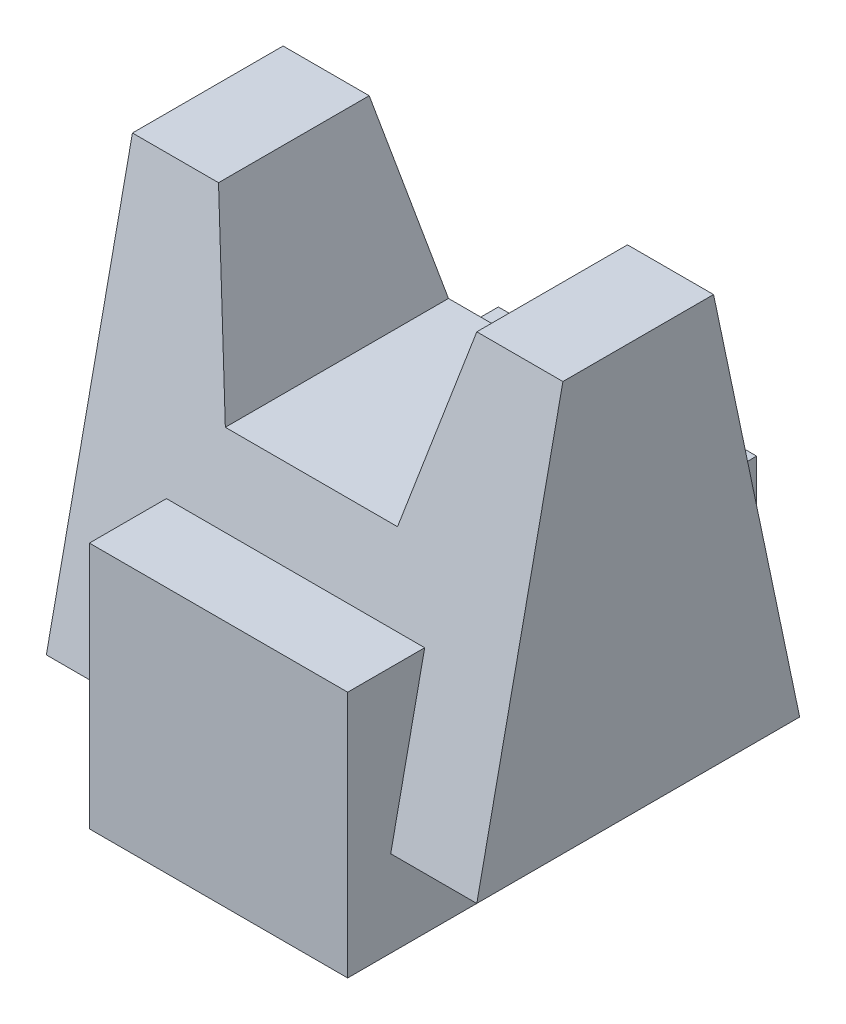
ISO-10303-21;
HEADER;
FILE_DESCRIPTION(('STEP AP214'),'2;1');
FILE_NAME('part.step','',(''),(''),'','','');
FILE_SCHEMA(('AUTOMOTIVE_DESIGN { 1 0 10303 214 1 1 1 1 }'));
ENDSEC;
DATA;
#1=APPLICATION_CONTEXT('core data for automotive mechanical design processes');
#2=APPLICATION_PROTOCOL_DEFINITION('international standard','automotive_design',2000,#1);
#3=PRODUCT_CONTEXT('',#1,'mechanical');
#4=PRODUCT('Part','Part','',(#3));
#5=PRODUCT_RELATED_PRODUCT_CATEGORY('part','',(#4));
#6=PRODUCT_DEFINITION_FORMATION('','',#4);
#7=PRODUCT_DEFINITION_CONTEXT('part definition',#1,'design');
#8=PRODUCT_DEFINITION('design','',#6,#7);
#9=PRODUCT_DEFINITION_SHAPE('','',#8);
#10=(LENGTH_UNIT() NAMED_UNIT(*) SI_UNIT(.MILLI.,.METRE.));
#11=(NAMED_UNIT(*) PLANE_ANGLE_UNIT() SI_UNIT($,.RADIAN.));
#12=(NAMED_UNIT(*) SI_UNIT($,.STERADIAN.) SOLID_ANGLE_UNIT());
#13=UNCERTAINTY_MEASURE_WITH_UNIT(LENGTH_MEASURE(1.E-05),#10,'distance_accuracy_value','');
#14=(GEOMETRIC_REPRESENTATION_CONTEXT(3) GLOBAL_UNCERTAINTY_ASSIGNED_CONTEXT((#13)) GLOBAL_UNIT_ASSIGNED_CONTEXT((#10,
#11,#12)) REPRESENTATION_CONTEXT('',''));
#15=CARTESIAN_POINT('',(0.,0.,0.));
#16=DIRECTION('',(0.,0.,1.));
#17=DIRECTION('',(1.,0.,0.));
#18=AXIS2_PLACEMENT_3D('',#15,#16,#17);
#19=CARTESIAN_POINT('',(0.,0.,15.));
#20=DIRECTION('',(0.,1.,0.));
#21=DIRECTION('',(0.,0.,1.));
#22=AXIS2_PLACEMENT_3D('',#19,#20,#21);
#23=PLANE('',#22);
#24=DIRECTION('',(1.,0.,0.));
#25=VECTOR('',#24,1.);
#26=CARTESIAN_POINT('',(0.,0.,15.));
#27=LINE('',#26,#25);
#28=CARTESIAN_POINT('',(12.,0.,15.));
#29=VERTEX_POINT('',#28);
#30=CARTESIAN_POINT('',(20.,0.,15.));
#31=VERTEX_POINT('',#30);
#32=EDGE_CURVE('E243',#29,#31,#27,.T.);
#33=ORIENTED_EDGE('',*,*,#32,.F.);
#34=DIRECTION('',(0.,0.,-1.));
#35=VECTOR('',#34,1.);
#36=CARTESIAN_POINT('',(12.,0.,15.));
#37=LINE('',#36,#35);
#38=CARTESIAN_POINT('',(12.,0.,-15.));
#39=VERTEX_POINT('',#38);
#40=EDGE_CURVE('E205',#29,#39,#37,.T.);
#41=ORIENTED_EDGE('',*,*,#40,.T.);
#42=DIRECTION('',(1.,0.,0.));
#43=VECTOR('',#42,1.);
#44=CARTESIAN_POINT('',(0.,0.,-15.));
#45=LINE('',#44,#43);
#46=CARTESIAN_POINT('',(20.,0.,-15.));
#47=VERTEX_POINT('',#46);
#48=EDGE_CURVE('E237',#39,#47,#45,.T.);
#49=ORIENTED_EDGE('',*,*,#48,.T.);
#50=DIRECTION('',(0.,0.,-1.));
#51=VECTOR('',#50,1.);
#52=CARTESIAN_POINT('',(20.,0.,15.));
#53=LINE('',#52,#51);
#54=EDGE_CURVE('E255',#31,#47,#53,.T.);
#55=ORIENTED_EDGE('',*,*,#54,.F.);
#56=EDGE_LOOP('',(#33,#41,#49,#55));
#57=FACE_BOUND('',#56,.T.);
#58=ADVANCED_FACE('F41',(#57),#23,.F.);
#59=CARTESIAN_POINT('',(2.35294117647059,-0.588235294117647,15.));
#60=DIRECTION('',(-0.970142500145332,0.242535625036333,0.));
#61=DIRECTION('',(-0.242535625036333,-0.970142500145332,0.));
#62=AXIS2_PLACEMENT_3D('',#59,#60,#61);
#63=PLANE('',#62);
#64=DIRECTION('',(-0.237629989454199,-0.950519957816794,0.200109464803536));
#65=VECTOR('',#64,1.);
#66=CARTESIAN_POINT('',(2.35882997027999,-0.564680118880025,15.1188800250274));
#67=LINE('',#66,#65);
#68=CARTESIAN_POINT('',(12.,38.,7.));
#69=VERTEX_POINT('',#68);
#70=CARTESIAN_POINT('',(8.,22.,10.3684210526316));
#71=VERTEX_POINT('',#70);
#72=EDGE_CURVE('E240',#69,#71,#67,.T.);
#73=ORIENTED_EDGE('',*,*,#72,.F.);
#74=DIRECTION('',(0.,0.,-1.));
#75=VECTOR('',#74,1.);
#76=CARTESIAN_POINT('',(12.,38.,15.));
#77=LINE('',#76,#75);
#78=CARTESIAN_POINT('',(12.,38.,-7.));
#79=VERTEX_POINT('',#78);
#80=EDGE_CURVE('E245',#69,#79,#77,.T.);
#81=ORIENTED_EDGE('',*,*,#80,.T.);
#82=DIRECTION('',(-0.237629989454199,-0.950519957816794,-0.200109464803536));
#83=VECTOR('',#82,1.);
#84=CARTESIAN_POINT('',(3.78539027060848,5.14156108243391,-13.9175660879086));
#85=LINE('',#84,#83);
#86=CARTESIAN_POINT('',(8.,22.,-10.3684210526316));
#87=VERTEX_POINT('',#86);
#88=EDGE_CURVE('E226',#79,#87,#85,.T.);
#89=ORIENTED_EDGE('',*,*,#88,.T.);
#90=DIRECTION('',(0.,0.,-1.));
#91=VECTOR('',#90,1.);
#92=CARTESIAN_POINT('',(8.,22.,15.));
#93=LINE('',#92,#91);
#94=EDGE_CURVE('E269',#71,#87,#93,.T.);
#95=ORIENTED_EDGE('',*,*,#94,.F.);
#96=EDGE_LOOP('',(#73,#81,#89,#95));
#97=FACE_BOUND('',#96,.T.);
#98=ADVANCED_FACE('F43',(#97),#63,.T.);
#99=CARTESIAN_POINT('',(0.,22.,15.));
#100=DIRECTION('',(0.,-1.,0.));
#101=DIRECTION('',(0.,0.,-1.));
#102=AXIS2_PLACEMENT_3D('',#99,#100,#101);
#103=PLANE('',#102);
#104=DIRECTION('',(0.,0.,-1.));
#105=VECTOR('',#104,1.);
#106=CARTESIAN_POINT('',(-8.,22.,15.));
#107=LINE('',#106,#105);
#108=CARTESIAN_POINT('',(-8.,22.,10.3684210526316));
#109=VERTEX_POINT('',#108);
#110=CARTESIAN_POINT('',(-8.,22.,-10.3684210526316));
#111=VERTEX_POINT('',#110);
#112=EDGE_CURVE('E262',#109,#111,#107,.T.);
#113=ORIENTED_EDGE('',*,*,#112,.F.);
#114=DIRECTION('',(1.,0.,0.));
#115=VECTOR('',#114,1.);
#116=CARTESIAN_POINT('',(0.,22.,10.3684210526316));
#117=LINE('',#116,#115);
#118=EDGE_CURVE('E234',#109,#71,#117,.T.);
#119=ORIENTED_EDGE('',*,*,#118,.T.);
#120=ORIENTED_EDGE('',*,*,#94,.T.);
#121=DIRECTION('',(1.,0.,0.));
#122=VECTOR('',#121,1.);
#123=CARTESIAN_POINT('',(0.,22.,-10.3684210526316));
#124=LINE('',#123,#122);
#125=EDGE_CURVE('E228',#111,#87,#124,.T.);
#126=ORIENTED_EDGE('',*,*,#125,.F.);
#127=EDGE_LOOP('',(#113,#119,#120,#126));
#128=FACE_BOUND('',#127,.T.);
#129=ADVANCED_FACE('F305',(#128),#103,.F.);
#130=CARTESIAN_POINT('',(-2.35294117647059,-0.588235294117648,15.));
#131=DIRECTION('',(-0.970142500145332,-0.242535625036333,0.));
#132=DIRECTION('',(0.242535625036333,-0.970142500145332,0.));
#133=AXIS2_PLACEMENT_3D('',#130,#131,#132);
#134=PLANE('',#133);
#135=DIRECTION('',(0.,0.,-1.));
#136=VECTOR('',#135,1.);
#137=CARTESIAN_POINT('',(-12.,38.,15.));
#138=LINE('',#137,#136);
#139=CARTESIAN_POINT('',(-12.,38.,7.));
#140=VERTEX_POINT('',#139);
#141=CARTESIAN_POINT('',(-12.,38.,-7.));
#142=VERTEX_POINT('',#141);
#143=EDGE_CURVE('E261',#140,#142,#138,.T.);
#144=ORIENTED_EDGE('',*,*,#143,.F.);
#145=DIRECTION('',(0.237629989454198,-0.950519957816794,0.200109464803536));
#146=VECTOR('',#145,1.);
#147=CARTESIAN_POINT('',(-2.35882997028,-0.564680118880026,15.1188800250274));
#148=LINE('',#147,#146);
#149=EDGE_CURVE('E233',#140,#109,#148,.T.);
#150=ORIENTED_EDGE('',*,*,#149,.T.);
#151=ORIENTED_EDGE('',*,*,#112,.T.);
#152=DIRECTION('',(0.237629989454198,-0.950519957816794,-0.200109464803536));
#153=VECTOR('',#152,1.);
#154=CARTESIAN_POINT('',(-3.78539027060848,5.14156108243391,-13.9175660879086));
#155=LINE('',#154,#153);
#156=EDGE_CURVE('E218',#142,#111,#155,.T.);
#157=ORIENTED_EDGE('',*,*,#156,.F.);
#158=EDGE_LOOP('',(#144,#150,#151,#157));
#159=FACE_BOUND('',#158,.T.);
#160=ADVANCED_FACE('F310',(#159),#134,.F.);
#161=CARTESIAN_POINT('',(0.,38.,15.));
#162=DIRECTION('',(0.,1.,0.));
#163=DIRECTION('',(0.,0.,1.));
#164=AXIS2_PLACEMENT_3D('',#161,#162,#163);
#165=PLANE('',#164);
#166=DIRECTION('',(1.,0.,0.));
#167=VECTOR('',#166,1.);
#168=CARTESIAN_POINT('',(-20.,38.,7.));
#169=LINE('',#168,#167);
#170=CARTESIAN_POINT('',(-20.,38.,7.));
#171=VERTEX_POINT('',#170);
#172=EDGE_CURVE('E213',#171,#140,#169,.T.);
#173=ORIENTED_EDGE('',*,*,#172,.T.);
#174=ORIENTED_EDGE('',*,*,#143,.T.);
#175=DIRECTION('',(1.,0.,0.));
#176=VECTOR('',#175,1.);
#177=CARTESIAN_POINT('',(-20.,38.,-7.));
#178=LINE('',#177,#176);
#179=CARTESIAN_POINT('',(-20.,38.,-7.));
#180=VERTEX_POINT('',#179);
#181=EDGE_CURVE('E217',#180,#142,#178,.T.);
#182=ORIENTED_EDGE('',*,*,#181,.F.);
#183=DIRECTION('',(0.,0.,-1.));
#184=VECTOR('',#183,1.);
#185=CARTESIAN_POINT('',(-20.,38.,15.));
#186=LINE('',#185,#184);
#187=EDGE_CURVE('E259',#171,#180,#186,.T.);
#188=ORIENTED_EDGE('',*,*,#187,.F.);
#189=EDGE_LOOP('',(#173,#174,#182,#188));
#190=FACE_BOUND('',#189,.T.);
#191=ADVANCED_FACE('F309',(#190),#165,.T.);
#192=CARTESIAN_POINT('',(-20.,0.,15.));
#193=DIRECTION('',(1.,0.,0.));
#194=DIRECTION('',(0.,1.,0.));
#195=AXIS2_PLACEMENT_3D('',#192,#193,#194);
#196=PLANE('',#195);
#197=DIRECTION('',(0.,0.,-1.));
#198=VECTOR('',#197,1.);
#199=CARTESIAN_POINT('',(-20.,0.,15.));
#200=LINE('',#199,#198);
#201=CARTESIAN_POINT('',(-20.,0.,15.));
#202=VERTEX_POINT('',#201);
#203=CARTESIAN_POINT('',(-20.,0.,-15.));
#204=VERTEX_POINT('',#203);
#205=EDGE_CURVE('E253',#202,#204,#200,.T.);
#206=ORIENTED_EDGE('',*,*,#205,.F.);
#207=DIRECTION('',(0.,0.978549784986749,-0.206010481049842));
#208=VECTOR('',#207,1.);
#209=CARTESIAN_POINT('',(-20.,0.,15.));
#210=LINE('',#209,#208);
#211=EDGE_CURVE('E63',#202,#171,#210,.T.);
#212=ORIENTED_EDGE('',*,*,#211,.T.);
#213=ORIENTED_EDGE('',*,*,#187,.T.);
#214=DIRECTION('',(0.,0.978549784986749,0.206010481049842));
#215=VECTOR('',#214,1.);
#216=CARTESIAN_POINT('',(-20.,0.,-15.));
#217=LINE('',#216,#215);
#218=EDGE_CURVE('E223',#204,#180,#217,.T.);
#219=ORIENTED_EDGE('',*,*,#218,.F.);
#220=EDGE_LOOP('',(#206,#212,#213,#219));
#221=FACE_BOUND('',#220,.T.);
#222=ADVANCED_FACE('F313',(#221),#196,.F.);
#223=CARTESIAN_POINT('',(20.,0.,15.));
#224=DIRECTION('',(-1.,0.,0.));
#225=DIRECTION('',(0.,0.,1.));
#226=AXIS2_PLACEMENT_3D('',#223,#224,#225);
#227=PLANE('',#226);
#228=DIRECTION('',(0.,0.,-1.));
#229=VECTOR('',#228,1.);
#230=CARTESIAN_POINT('',(20.,38.,15.));
#231=LINE('',#230,#229);
#232=CARTESIAN_POINT('',(20.,38.,7.));
#233=VERTEX_POINT('',#232);
#234=CARTESIAN_POINT('',(20.,38.,-7.));
#235=VERTEX_POINT('',#234);
#236=EDGE_CURVE('E248',#233,#235,#231,.T.);
#237=ORIENTED_EDGE('',*,*,#236,.F.);
#238=DIRECTION('',(0.,0.978549784986749,-0.206010481049842));
#239=VECTOR('',#238,1.);
#240=CARTESIAN_POINT('',(20.,0.,15.));
#241=LINE('',#240,#239);
#242=EDGE_CURVE('E215',#31,#233,#241,.T.);
#243=ORIENTED_EDGE('',*,*,#242,.F.);
#244=ORIENTED_EDGE('',*,*,#54,.T.);
#245=DIRECTION('',(0.,0.978549784986749,0.206010481049842));
#246=VECTOR('',#245,1.);
#247=CARTESIAN_POINT('',(20.,0.,-15.));
#248=LINE('',#247,#246);
#249=EDGE_CURVE('E211',#47,#235,#248,.T.);
#250=ORIENTED_EDGE('',*,*,#249,.T.);
#251=EDGE_LOOP('',(#237,#243,#244,#250));
#252=FACE_BOUND('',#251,.T.);
#253=ADVANCED_FACE('F292',(#252),#227,.F.);
#254=CARTESIAN_POINT('',(0.,38.,15.));
#255=DIRECTION('',(0.,-1.,0.));
#256=DIRECTION('',(0.,0.,-1.));
#257=AXIS2_PLACEMENT_3D('',#254,#255,#256);
#258=PLANE('',#257);
#259=ORIENTED_EDGE('',*,*,#80,.F.);
#260=EDGE_CURVE('E212',#69,#233,#169,.T.);
#261=ORIENTED_EDGE('',*,*,#260,.T.);
#262=ORIENTED_EDGE('',*,*,#236,.T.);
#263=EDGE_CURVE('E209',#79,#235,#178,.T.);
#264=ORIENTED_EDGE('',*,*,#263,.F.);
#265=EDGE_LOOP('',(#259,#261,#262,#264));
#266=FACE_BOUND('',#265,.T.);
#267=ADVANCED_FACE('F300',(#266),#258,.F.);
#268=CARTESIAN_POINT('',(-12.,0.,-15.));
#269=VERTEX_POINT('',#268);
#270=EDGE_CURVE('E242',#204,#269,#45,.T.);
#271=ORIENTED_EDGE('',*,*,#270,.T.);
#272=DIRECTION('',(0.,0.,1.));
#273=VECTOR('',#272,1.);
#274=CARTESIAN_POINT('',(-12.,0.,15.));
#275=LINE('',#274,#273);
#276=CARTESIAN_POINT('',(-12.,0.,15.));
#277=VERTEX_POINT('',#276);
#278=EDGE_CURVE('E195',#269,#277,#275,.T.);
#279=ORIENTED_EDGE('',*,*,#278,.T.);
#280=EDGE_CURVE('E239',#202,#277,#27,.T.);
#281=ORIENTED_EDGE('',*,*,#280,.F.);
#282=ORIENTED_EDGE('',*,*,#205,.T.);
#283=EDGE_LOOP('',(#271,#279,#281,#282));
#284=FACE_BOUND('',#283,.T.);
#285=ADVANCED_FACE('F320',(#284),#23,.F.);
#286=CARTESIAN_POINT('',(-20.,0.,-15.));
#287=DIRECTION('',(0.,0.206010481049842,-0.978549784986749));
#288=DIRECTION('',(0.,0.978549784986749,0.206010481049842));
#289=AXIS2_PLACEMENT_3D('',#286,#287,#288);
#290=PLANE('',#289);
#291=DIRECTION('',(0.,-0.978549784986749,-0.206010481049842));
#292=VECTOR('',#291,1.);
#293=CARTESIAN_POINT('',(12.,0.,-15.));
#294=LINE('',#293,#292);
#295=CARTESIAN_POINT('',(12.,15.,-11.8421052631579));
#296=VERTEX_POINT('',#295);
#297=EDGE_CURVE('E210',#296,#39,#294,.T.);
#298=ORIENTED_EDGE('',*,*,#297,.F.);
#299=DIRECTION('',(1.,0.,0.));
#300=VECTOR('',#299,1.);
#301=CARTESIAN_POINT('',(-20.,15.,-11.8421052631579));
#302=LINE('',#301,#300);
#303=CARTESIAN_POINT('',(-12.,15.,-11.8421052631579));
#304=VERTEX_POINT('',#303);
#305=EDGE_CURVE('E204',#304,#296,#302,.T.);
#306=ORIENTED_EDGE('',*,*,#305,.F.);
#307=DIRECTION('',(0.,0.978549784986749,0.206010481049842));
#308=VECTOR('',#307,1.);
#309=CARTESIAN_POINT('',(-12.,0.,-15.));
#310=LINE('',#309,#308);
#311=EDGE_CURVE('E199',#269,#304,#310,.T.);
#312=ORIENTED_EDGE('',*,*,#311,.F.);
#313=ORIENTED_EDGE('',*,*,#270,.F.);
#314=ORIENTED_EDGE('',*,*,#218,.T.);
#315=ORIENTED_EDGE('',*,*,#181,.T.);
#316=ORIENTED_EDGE('',*,*,#156,.T.);
#317=ORIENTED_EDGE('',*,*,#125,.T.);
#318=ORIENTED_EDGE('',*,*,#88,.F.);
#319=ORIENTED_EDGE('',*,*,#263,.T.);
#320=ORIENTED_EDGE('',*,*,#249,.F.);
#321=ORIENTED_EDGE('',*,*,#48,.F.);
#322=EDGE_LOOP('',(#298,#306,#312,#313,#314,#315,#316,#317,#318,#319,#320,#321));
#323=FACE_BOUND('',#322,.T.);
#324=ADVANCED_FACE('F288',(#323),#290,.T.);
#325=CARTESIAN_POINT('',(-20.,0.,15.));
#326=DIRECTION('',(0.,-0.206010481049842,-0.978549784986749));
#327=DIRECTION('',(0.,0.978549784986749,-0.206010481049842));
#328=AXIS2_PLACEMENT_3D('',#325,#326,#327);
#329=PLANE('',#328);
#330=DIRECTION('',(1.,0.,0.));
#331=VECTOR('',#330,1.);
#332=CARTESIAN_POINT('',(-20.,15.,11.8421052631579));
#333=LINE('',#332,#331);
#334=CARTESIAN_POINT('',(-12.,15.,11.8421052631579));
#335=VERTEX_POINT('',#334);
#336=CARTESIAN_POINT('',(12.,15.,11.8421052631579));
#337=VERTEX_POINT('',#336);
#338=EDGE_CURVE('E47',#335,#337,#333,.T.);
#339=ORIENTED_EDGE('',*,*,#338,.T.);
#340=DIRECTION('',(0.,-0.978549784986749,0.206010481049842));
#341=VECTOR('',#340,1.);
#342=CARTESIAN_POINT('',(12.,0.,15.));
#343=LINE('',#342,#341);
#344=EDGE_CURVE('E11',#337,#29,#343,.T.);
#345=ORIENTED_EDGE('',*,*,#344,.T.);
#346=ORIENTED_EDGE('',*,*,#32,.T.);
#347=ORIENTED_EDGE('',*,*,#242,.T.);
#348=ORIENTED_EDGE('',*,*,#260,.F.);
#349=ORIENTED_EDGE('',*,*,#72,.T.);
#350=ORIENTED_EDGE('',*,*,#118,.F.);
#351=ORIENTED_EDGE('',*,*,#149,.F.);
#352=ORIENTED_EDGE('',*,*,#172,.F.);
#353=ORIENTED_EDGE('',*,*,#211,.F.);
#354=ORIENTED_EDGE('',*,*,#280,.T.);
#355=DIRECTION('',(0.,0.978549784986749,-0.206010481049842));
#356=VECTOR('',#355,1.);
#357=CARTESIAN_POINT('',(-12.,0.,15.));
#358=LINE('',#357,#356);
#359=EDGE_CURVE('E266',#277,#335,#358,.T.);
#360=ORIENTED_EDGE('',*,*,#359,.T.);
#361=EDGE_LOOP('',(#339,#345,#346,#347,#348,#349,#350,#351,#352,#353,#354,#360));
#362=FACE_BOUND('',#361,.T.);
#363=ADVANCED_FACE('F271',(#362),#329,.F.);
#364=CARTESIAN_POINT('',(-12.,15.,19.));
#365=DIRECTION('',(0.,1.,0.));
#366=DIRECTION('',(-1.,0.,0.));
#367=AXIS2_PLACEMENT_3D('',#364,#365,#366);
#368=PLANE('',#367);
#369=ORIENTED_EDGE('',*,*,#338,.F.);
#370=DIRECTION('',(0.,0.,-1.));
#371=VECTOR('',#370,1.);
#372=CARTESIAN_POINT('',(-12.,15.,19.));
#373=LINE('',#372,#371);
#374=CARTESIAN_POINT('',(-12.,15.,19.));
#375=VERTEX_POINT('',#374);
#376=EDGE_CURVE('E57',#375,#335,#373,.T.);
#377=ORIENTED_EDGE('',*,*,#376,.F.);
#378=DIRECTION('',(1.,0.,0.));
#379=VECTOR('',#378,1.);
#380=CARTESIAN_POINT('',(-12.,15.,19.));
#381=LINE('',#380,#379);
#382=CARTESIAN_POINT('',(12.,15.,19.));
#383=VERTEX_POINT('',#382);
#384=EDGE_CURVE('E172',#375,#383,#381,.T.);
#385=ORIENTED_EDGE('',*,*,#384,.T.);
#386=DIRECTION('',(0.,0.,-1.));
#387=VECTOR('',#386,1.);
#388=CARTESIAN_POINT('',(12.,15.,19.));
#389=LINE('',#388,#387);
#390=EDGE_CURVE('E194',#383,#337,#389,.T.);
#391=ORIENTED_EDGE('',*,*,#390,.T.);
#392=EDGE_LOOP('',(#369,#377,#385,#391));
#393=FACE_BOUND('',#392,.T.);
#394=ADVANCED_FACE('F277',(#393),#368,.T.);
#395=CARTESIAN_POINT('',(12.,-8.,19.));
#396=DIRECTION('',(0.,-1.,0.));
#397=DIRECTION('',(1.,0.,0.));
#398=AXIS2_PLACEMENT_3D('',#395,#396,#397);
#399=PLANE('',#398);
#400=DIRECTION('',(-1.,0.,0.));
#401=VECTOR('',#400,1.);
#402=CARTESIAN_POINT('',(12.,-8.,-19.));
#403=LINE('',#402,#401);
#404=CARTESIAN_POINT('',(12.,-8.,-19.));
#405=VERTEX_POINT('',#404);
#406=CARTESIAN_POINT('',(-12.,-8.,-19.));
#407=VERTEX_POINT('',#406);
#408=EDGE_CURVE('E187',#405,#407,#403,.T.);
#409=ORIENTED_EDGE('',*,*,#408,.F.);
#410=DIRECTION('',(0.,0.,-1.));
#411=VECTOR('',#410,1.);
#412=CARTESIAN_POINT('',(12.,-8.,19.));
#413=LINE('',#412,#411);
#414=CARTESIAN_POINT('',(12.,-8.,19.));
#415=VERTEX_POINT('',#414);
#416=EDGE_CURVE('E180',#415,#405,#413,.T.);
#417=ORIENTED_EDGE('',*,*,#416,.F.);
#418=DIRECTION('',(-1.,0.,0.));
#419=VECTOR('',#418,1.);
#420=CARTESIAN_POINT('',(12.,-8.,19.));
#421=LINE('',#420,#419);
#422=CARTESIAN_POINT('',(-12.,-8.,19.));
#423=VERTEX_POINT('',#422);
#424=EDGE_CURVE('E171',#415,#423,#421,.T.);
#425=ORIENTED_EDGE('',*,*,#424,.T.);
#426=DIRECTION('',(0.,0.,-1.));
#427=VECTOR('',#426,1.);
#428=CARTESIAN_POINT('',(-12.,-8.,19.));
#429=LINE('',#428,#427);
#430=EDGE_CURVE('E153',#423,#407,#429,.T.);
#431=ORIENTED_EDGE('',*,*,#430,.T.);
#432=EDGE_LOOP('',(#409,#417,#425,#431));
#433=FACE_BOUND('',#432,.T.);
#434=ADVANCED_FACE('F176',(#433),#399,.T.);
#435=CARTESIAN_POINT('',(12.,15.,19.));
#436=DIRECTION('',(1.,0.,0.));
#437=DIRECTION('',(0.,1.,0.));
#438=AXIS2_PLACEMENT_3D('',#435,#436,#437);
#439=PLANE('',#438);
#440=CARTESIAN_POINT('',(12.,15.,-19.));
#441=VERTEX_POINT('',#440);
#442=EDGE_CURVE('E196',#296,#441,#389,.T.);
#443=ORIENTED_EDGE('',*,*,#442,.F.);
#444=ORIENTED_EDGE('',*,*,#297,.T.);
#445=ORIENTED_EDGE('',*,*,#40,.F.);
#446=ORIENTED_EDGE('',*,*,#344,.F.);
#447=ORIENTED_EDGE('',*,*,#390,.F.);
#448=DIRECTION('',(0.,-1.,0.));
#449=VECTOR('',#448,1.);
#450=CARTESIAN_POINT('',(12.,15.,19.));
#451=LINE('',#450,#449);
#452=EDGE_CURVE('E165',#383,#415,#451,.T.);
#453=ORIENTED_EDGE('',*,*,#452,.T.);
#454=ORIENTED_EDGE('',*,*,#416,.T.);
#455=DIRECTION('',(0.,-1.,0.));
#456=VECTOR('',#455,1.);
#457=CARTESIAN_POINT('',(12.,15.,-19.));
#458=LINE('',#457,#456);
#459=EDGE_CURVE('E178',#441,#405,#458,.T.);
#460=ORIENTED_EDGE('',*,*,#459,.F.);
#461=EDGE_LOOP('',(#443,#444,#445,#446,#447,#453,#454,#460));
#462=FACE_BOUND('',#461,.T.);
#463=ADVANCED_FACE('F276',(#462),#439,.T.);
#464=CARTESIAN_POINT('',(-12.,15.,-19.));
#465=VERTEX_POINT('',#464);
#466=EDGE_CURVE('E161',#304,#465,#373,.T.);
#467=ORIENTED_EDGE('',*,*,#466,.F.);
#468=ORIENTED_EDGE('',*,*,#305,.T.);
#469=ORIENTED_EDGE('',*,*,#442,.T.);
#470=DIRECTION('',(1.,0.,0.));
#471=VECTOR('',#470,1.);
#472=CARTESIAN_POINT('',(-12.,15.,-19.));
#473=LINE('',#472,#471);
#474=EDGE_CURVE('E181',#465,#441,#473,.T.);
#475=ORIENTED_EDGE('',*,*,#474,.F.);
#476=EDGE_LOOP('',(#467,#468,#469,#475));
#477=FACE_BOUND('',#476,.T.);
#478=ADVANCED_FACE('F322',(#477),#368,.T.);
#479=CARTESIAN_POINT('',(-12.,-8.,19.));
#480=DIRECTION('',(-1.,0.,0.));
#481=DIRECTION('',(0.,0.,1.));
#482=AXIS2_PLACEMENT_3D('',#479,#480,#481);
#483=PLANE('',#482);
#484=ORIENTED_EDGE('',*,*,#278,.F.);
#485=ORIENTED_EDGE('',*,*,#311,.T.);
#486=ORIENTED_EDGE('',*,*,#466,.T.);
#487=DIRECTION('',(0.,1.,0.));
#488=VECTOR('',#487,1.);
#489=CARTESIAN_POINT('',(-12.,-8.,-19.));
#490=LINE('',#489,#488);
#491=EDGE_CURVE('E157',#407,#465,#490,.T.);
#492=ORIENTED_EDGE('',*,*,#491,.F.);
#493=ORIENTED_EDGE('',*,*,#430,.F.);
#494=DIRECTION('',(0.,1.,0.));
#495=VECTOR('',#494,1.);
#496=CARTESIAN_POINT('',(-12.,-8.,19.));
#497=LINE('',#496,#495);
#498=EDGE_CURVE('E158',#423,#375,#497,.T.);
#499=ORIENTED_EDGE('',*,*,#498,.T.);
#500=ORIENTED_EDGE('',*,*,#376,.T.);
#501=ORIENTED_EDGE('',*,*,#359,.F.);
#502=EDGE_LOOP('',(#484,#485,#486,#492,#493,#499,#500,#501));
#503=FACE_BOUND('',#502,.T.);
#504=ADVANCED_FACE('F154',(#503),#483,.T.);
#505=CARTESIAN_POINT('',(0.,0.,19.));
#506=DIRECTION('',(0.,0.,-1.));
#507=DIRECTION('',(-1.,0.,0.));
#508=AXIS2_PLACEMENT_3D('',#505,#506,#507);
#509=PLANE('',#508);
#510=ORIENTED_EDGE('',*,*,#424,.F.);
#511=ORIENTED_EDGE('',*,*,#452,.F.);
#512=ORIENTED_EDGE('',*,*,#384,.F.);
#513=ORIENTED_EDGE('',*,*,#498,.F.);
#514=EDGE_LOOP('',(#510,#511,#512,#513));
#515=FACE_BOUND('',#514,.T.);
#516=ADVANCED_FACE('F169',(#515),#509,.F.);
#517=CARTESIAN_POINT('',(0.,0.,-19.));
#518=DIRECTION('',(0.,0.,-1.));
#519=DIRECTION('',(-1.,0.,0.));
#520=AXIS2_PLACEMENT_3D('',#517,#518,#519);
#521=PLANE('',#520);
#522=ORIENTED_EDGE('',*,*,#408,.T.);
#523=ORIENTED_EDGE('',*,*,#491,.T.);
#524=ORIENTED_EDGE('',*,*,#474,.T.);
#525=ORIENTED_EDGE('',*,*,#459,.T.);
#526=EDGE_LOOP('',(#522,#523,#524,#525));
#527=FACE_BOUND('',#526,.T.);
#528=ADVANCED_FACE('F323',(#527),#521,.T.);
#529=CLOSED_SHELL('',(#58,#98,#129,#160,#191,#222,#253,#267,#285,#324,#363,#394,#434,#463,#478,
#504,#516,#528));
#530=MANIFOLD_SOLID_BREP('B2',#529);
#531=ADVANCED_BREP_SHAPE_REPRESENTATION('',(#18,#530),#14);
#532=SHAPE_DEFINITION_REPRESENTATION(#9,#531);
ENDSEC;
END-ISO-10303-21;
